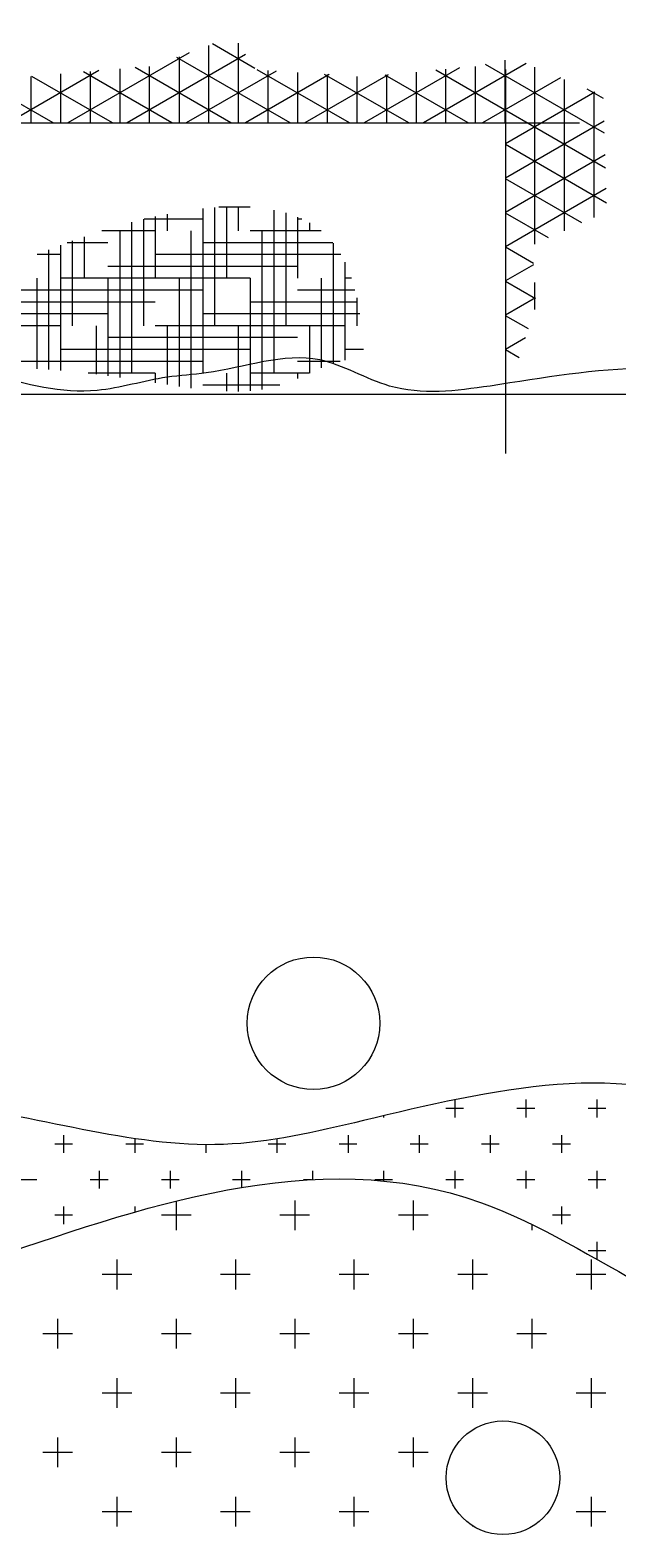
# Model space of a CAD drawing. Units: inches. Extents: x 3731 to 4318, y 1310 to 2388.
# Tile 45 of 57: x 4167 to 4192, y 1977 to 2043. Entities that reach past the tile are written whole.
import ezdxf

# ---------------------------------------------------------------- set-up
doc = ezdxf.new("R2010")
doc.units = ezdxf.units.IN
doc.layers.add('A-ANNO-DIMS', color=2, linetype='Continuous', lineweight=18)
doc.layers.add('A-FURN', color=8, linetype='Continuous', lineweight=13)
doc.styles.get("Standard").update_dxf_attribs({"font": 'arial.ttf'})
doc.dimstyles.get("Standard").update_dxf_attribs({"dimtxt": 0.18, "dimasz": 0.18, "dimexe": 0.18, "dimexo": 0.0625, "dimgap": 0.09, "dimtad": 0, "dimtih": 1, "dimtoh": 1, "dimdec": 4, "dimzin": 0, "dimdsep": 46, "dimtxsty": 'Standard', "dimcen": 0.09, "dimadec": 0, "dimazin": 0, "dimtfac": 1, "dimtdec": 4, "dimtofl": 0, "dimtmove": 0, "dimatfit": 3, "dimfxl": 1, "dimtolj": 1, "dimtzin": 0, "dimarcsym": 0})

# ---------------------------------------------------------------- blocks, each defined once
blk = doc.blocks.new('A$C200C7901')
at = {"linetype": 'ByBlock'}
for p, q in [((0.9504, 1.532), (0.9504, 1.5633)), ((0.9504, 1.532), (0.9504, 1.5633)), ((1.2004, 1.532), (1.2004, 1.5633)), ((1.2004, 1.532), (1.2004, 1.5633)), ((1.3254, 1.532), (1.3254, 1.5633)), ((1.3254, 1.532), (1.3254, 1.5633)), ((1.4504, 1.532), (1.4504, 1.5633)), ((1.4504, 1.532), (1.4504, 1.5633)), ((0.9347, 1.5477), (0.966, 1.5477)), ((0.9347, 1.5477), (0.966, 1.5477)), ((1.1847, 1.5477), (1.216, 1.5477)), ((1.1847, 1.5477), (1.216, 1.5477)), ((1.3097, 1.5477), (1.341, 1.5477)), ((1.3097, 1.5477), (1.341, 1.5477)), ((1.4347, 1.5477), (1.466, 1.5477)), ((1.4347, 1.5477), (1.466, 1.5477)), ((1.1379, 1.4695), (1.1379, 1.5008)), ((1.1379, 1.4695), (1.1379, 1.5008)), ((1.2629, 1.4695), (1.2629, 1.5008)), ((1.2629, 1.4695), (1.2629, 1.5008)), ((1.3879, 1.4695), (1.3879, 1.5008)), ((1.3879, 1.4695), (1.3879, 1.5008)), ((1.5129, 1.4695), (1.5129, 1.5008)), ((1.5129, 1.4695), (1.5129, 1.5008)), ((1.1222, 1.4852), (1.1535, 1.4852)), ((1.1222, 1.4852), (1.1535, 1.4852)), ((1.2472, 1.4852), (1.2785, 1.4852)), ((1.2472, 1.4852), (1.2785, 1.4852)), ((1.3722, 1.4852), (1.4035, 1.4852)), ((1.3722, 1.4852), (1.4035, 1.4852)), ((1.4972, 1.4852), (1.5285, 1.4852)), ((1.4972, 1.4852), (1.5285, 1.4852)), ((0.9504, 1.407), (0.9504, 1.4383)), ((0.9504, 1.407), (0.9504, 1.4383)), ((1.0754, 1.407), (1.0754, 1.4383)), ((1.0754, 1.407), (1.0754, 1.4383)), ((1.2004, 1.407), (1.2004, 1.4383)), ((1.2004, 1.407), (1.2004, 1.4383)), ((1.3254, 1.407), (1.3254, 1.4383)), ((1.3254, 1.407), (1.3254, 1.4383)), ((1.4504, 1.407), (1.4504, 1.4383)), ((1.4504, 1.407), (1.4504, 1.4383)), ((0.9347, 1.4227), (0.966, 1.4227)), ((0.9347, 1.4227), (0.966, 1.4227)), ((1.0597, 1.4227), (1.091, 1.4227)), ((1.0597, 1.4227), (1.091, 1.4227)), ((1.1847, 1.4227), (1.216, 1.4227)), ((1.1847, 1.4227), (1.216, 1.4227)), ((1.3097, 1.4227), (1.341, 1.4227)), ((1.3097, 1.4227), (1.341, 1.4227)), ((1.4347, 1.4227), (1.466, 1.4227)), ((1.4347, 1.4227), (1.466, 1.4227)), ((1.0129, 1.3445), (1.0129, 1.3758)), ((1.0129, 1.3445), (1.0129, 1.3758)), ((1.1379, 1.3445), (1.1379, 1.3758)), ((1.1379, 1.3445), (1.1379, 1.3758)), ((1.2629, 1.3445), (1.2629, 1.3758)), ((1.2629, 1.3445), (1.2629, 1.3758)), ((1.3879, 1.3445), (1.3879, 1.3758)), ((1.3879, 1.3445), (1.3879, 1.3758)), ((1.5129, 1.3445), (1.5129, 1.3758)), ((1.5129, 1.3445), (1.5129, 1.3758)), ((0.9972, 1.3602), (1.0285, 1.3602)), ((0.9972, 1.3602), (1.0285, 1.3602)), ((1.1222, 1.3602), (1.1535, 1.3602)), ((1.1222, 1.3602), (1.1535, 1.3602)), ((1.2472, 1.3602), (1.2785, 1.3602)), ((1.2472, 1.3602), (1.2785, 1.3602)), ((1.3722, 1.3602), (1.4035, 1.3602)), ((1.3722, 1.3602), (1.4035, 1.3602)), ((1.4972, 1.3602), (1.5285, 1.3602)), ((1.4972, 1.3602), (1.5285, 1.3602)), ((0.9504, 1.282), (0.9504, 1.3133)), ((0.9504, 1.282), (0.9504, 1.3133)), ((1.0754, 1.282), (1.0754, 1.3133)), ((1.0754, 1.282), (1.0754, 1.3133)), ((1.2004, 1.282), (1.2004, 1.3133)), ((1.2004, 1.282), (1.2004, 1.3133)), ((1.3254, 1.282), (1.3254, 1.3133)), ((1.3254, 1.282), (1.3254, 1.3133)), ((1.4504, 1.282), (1.4504, 1.3133)), ((1.4504, 1.282), (1.4504, 1.3133)), ((0.9347, 1.2977), (0.966, 1.2977)), ((0.9347, 1.2977), (0.966, 1.2977)), ((1.0597, 1.2977), (1.091, 1.2977)), ((1.0597, 1.2977), (1.091, 1.2977)), ((1.1847, 1.2977), (1.216, 1.2977)), ((1.1847, 1.2977), (1.216, 1.2977)), ((1.3097, 1.2977), (1.341, 1.2977)), ((1.3097, 1.2977), (1.341, 1.2977)), ((1.4347, 1.2977), (1.466, 1.2977)), ((1.4347, 1.2977), (1.466, 1.2977)), ((0.9347, 1.2727), (0.9535, 1.2727)), ((0.9347, 1.2727), (0.9535, 1.2727)), ((0.9441, 1.2633), (0.9441, 1.2816)), ((0.9441, 1.2633), (0.9441, 1.2816)), ((0.9816, 1.2258), (0.9816, 1.2445)), ((0.9816, 1.2258), (0.9816, 1.2445)), ((1.0129, 1.2448), (1.0129, 1.2508)), ((1.0129, 1.2448), (1.0129, 1.2508)), ((1.1379, 1.2195), (1.1379, 1.2508)), ((1.1379, 1.2195), (1.1379, 1.2508)), ((1.2629, 1.2195), (1.2629, 1.2508)), ((1.2629, 1.2195), (1.2629, 1.2508)), ((1.3879, 1.2202), (1.3879, 1.2508)), ((1.3879, 1.2202), (1.3879, 1.2508)), ((1.5066, 1.2258), (1.5066, 1.2445)), ((1.5066, 1.2258), (1.5066, 1.2445)), ((0.9722, 1.2352), (0.991, 1.2352)), ((0.9722, 1.2352), (0.991, 1.2352)), ((1.1222, 1.2352), (1.1535, 1.2352)), ((1.1222, 1.2352), (1.1535, 1.2352)), ((1.2472, 1.2352), (1.2785, 1.2352)), ((1.2472, 1.2352), (1.2785, 1.2352)), ((1.3722, 1.2352), (1.4035, 1.2352)), ((1.3722, 1.2352), (1.4035, 1.2352)), ((1.4316, 1.2258), (1.4316, 1.2318)), ((1.4316, 1.2258), (1.4316, 1.2318)), ((1.4972, 1.2352), (1.516, 1.2352)), ((1.4972, 1.2352), (1.516, 1.2352)), ((0.9347, 1.1977), (0.9535, 1.1977)), ((0.9347, 1.1977), (0.9535, 1.1977)), ((0.9441, 1.1883), (0.9441, 1.207)), ((0.9441, 1.1883), (0.9441, 1.207)), ((1.0097, 1.1977), (1.0285, 1.1977)), ((1.0097, 1.1977), (1.0285, 1.1977)), ((1.0191, 1.1883), (1.0191, 1.207)), ((1.0191, 1.1883), (1.0191, 1.207)), ((1.0847, 1.1977), (1.1035, 1.1977)), ((1.0847, 1.1977), (1.1035, 1.1977)), ((1.0941, 1.1883), (1.0941, 1.207)), ((1.0941, 1.1883), (1.0941, 1.207)), ((1.1597, 1.1977), (1.1785, 1.1977)), ((1.1597, 1.1977), (1.1785, 1.1977)), ((1.1691, 1.1883), (1.1691, 1.1991)), ((1.1691, 1.1883), (1.1691, 1.1991)), ((1.2441, 1.1883), (1.2441, 1.1976)), ((1.2441, 1.1883), (1.2441, 1.1976)), ((1.2452, 1.1977), (1.2535, 1.1977)), ((1.2452, 1.1977), (1.2535, 1.1977)), ((1.3097, 1.1977), (1.3285, 1.1977)), ((1.3097, 1.1977), (1.3285, 1.1977)), ((1.3191, 1.1883), (1.3191, 1.2059)), ((1.3191, 1.1883), (1.3191, 1.2059)), ((1.3847, 1.1977), (1.4035, 1.1977)), ((1.3847, 1.1977), (1.4035, 1.1977)), ((1.3941, 1.1883), (1.3941, 1.207)), ((1.3941, 1.1883), (1.3941, 1.207)), ((1.4597, 1.1977), (1.4785, 1.1977)), ((1.4597, 1.1977), (1.4785, 1.1977)), ((1.4691, 1.1883), (1.4691, 1.207)), ((1.4691, 1.1883), (1.4691, 1.207)), ((1.5347, 1.1977), (1.5535, 1.1977)), ((1.5347, 1.1977), (1.5535, 1.1977)), ((0.9722, 1.1602), (0.991, 1.1602)), ((0.9722, 1.1602), (0.991, 1.1602)), ((0.9816, 1.1508), (0.9816, 1.1695)), ((0.9816, 1.1508), (0.9816, 1.1695)), ((1.0472, 1.1602), (1.066, 1.1602)), ((1.0472, 1.1602), (1.066, 1.1602)), ((1.0566, 1.1508), (1.0566, 1.1695)), ((1.0566, 1.1508), (1.0566, 1.1695)), ((1.1222, 1.1602), (1.141, 1.1602)), ((1.1222, 1.1602), (1.141, 1.1602)), ((1.1316, 1.1508), (1.1316, 1.1695)), ((1.1316, 1.1508), (1.1316, 1.1695)), ((1.1972, 1.1602), (1.216, 1.1602)), ((1.1972, 1.1602), (1.216, 1.1602)), ((1.2066, 1.1508), (1.2066, 1.1695)), ((1.2066, 1.1508), (1.2066, 1.1695)), ((1.2722, 1.1602), (1.291, 1.1602)), ((1.2722, 1.1602), (1.291, 1.1602)), ((1.2816, 1.1547), (1.2816, 1.1695)), ((1.2816, 1.1547), (1.2816, 1.1695)), ((1.3566, 1.1608), (1.3566, 1.1695)), ((1.3566, 1.1608), (1.3566, 1.1695)), ((1.4222, 1.1602), (1.441, 1.1602)), ((1.4222, 1.1602), (1.441, 1.1602)), ((1.4316, 1.1544), (1.4316, 1.1695)), ((1.4316, 1.1544), (1.4316, 1.1695)), ((1.4972, 1.1602), (1.516, 1.1602)), ((1.4972, 1.1602), (1.516, 1.1602)), ((1.5066, 1.1508), (1.5066, 1.1695)), ((1.5066, 1.1508), (1.5066, 1.1695)), ((0.9441, 1.1133), (0.9441, 1.132)), ((0.9441, 1.1133), (0.9441, 1.132)), ((1.0191, 1.1133), (1.0191, 1.132)), ((1.0191, 1.1133), (1.0191, 1.132)), ((1.0941, 1.1136), (1.0941, 1.132)), ((1.0941, 1.1136), (1.0941, 1.132)), ((1.1691, 1.1303), (1.1691, 1.132)), ((1.1691, 1.1303), (1.1691, 1.132)), ((0.9347, 1.1227), (0.9535, 1.1227)), ((0.9347, 1.1227), (0.9535, 1.1227)), ((1.0097, 1.1227), (1.0285, 1.1227)), ((1.0097, 1.1227), (1.0285, 1.1227)), ((1.0847, 1.1227), (1.1035, 1.1227)), ((1.0847, 1.1227), (1.1035, 1.1227)), ((1.3099, 0.2477), (1.3099, 0.3663)), ((1.3099, 0.2477), (1.3099, 0.3663)), ((1.3224, 0.2977), (1.3224, 0.3669)), ((1.3224, 0.2977), (1.3224, 0.3669)), ((1.3349, 0.3477), (1.3349, 0.3668)), ((1.3349, 0.3477), (1.3349, 0.3668)), ((1.2599, 0.3477), (1.2599, 0.3531)), ((1.2599, 0.3477), (1.2599, 0.3531)), ((1.2785, 0.3602), (1.3599, 0.3602)), ((1.2785, 0.3602), (1.3599, 0.3602)), ((1.2974, 0.1977), (1.2974, 0.3647)), ((1.2974, 0.1977), (1.2974, 0.3647)), ((1.3724, 0.1977), (1.3724, 0.3634)), ((1.3724, 0.1977), (1.3724, 0.3634)), ((1.3849, 0.2477), (1.3849, 0.3616)), ((1.3849, 0.2477), (1.3849, 0.3616)), ((1.3974, 0.2977), (1.3974, 0.3597)), ((1.3974, 0.2977), (1.3974, 0.3597)), ((1.4099, 0.3477), (1.4099, 0.3578)), ((1.4099, 0.3477), (1.4099, 0.3578)), ((1.4474, 0.1977), (1.4474, 0.3521)), ((1.4474, 0.1977), (1.4474, 0.3521)), ((1.4599, 0.2477), (1.4599, 0.3504)), ((1.4599, 0.2477), (1.4599, 0.3504)), ((1.2099, 0.2308), (1.2099, 0.334)), ((1.2099, 0.2308), (1.2099, 0.334)), ((1.2148, 0.3352), (1.2599, 0.3352)), ((1.2148, 0.3352), (1.2599, 0.3352)), ((1.2224, 0.2106), (1.2224, 0.3375)), ((1.2224, 0.2106), (1.2224, 0.3375)), ((1.2349, 0.2477), (1.2349, 0.3422)), ((1.2349, 0.2477), (1.2349, 0.3422)), ((1.2474, 0.2977), (1.2474, 0.3476)), ((1.2474, 0.2977), (1.2474, 0.3476)), ((1.2475, 0.3477), (1.3099, 0.3477)), ((1.2475, 0.3477), (1.3099, 0.3477)), ((1.2849, 0.1758), (1.2849, 0.3477)), ((1.2849, 0.1758), (1.2849, 0.3477)), ((1.3599, 0.1741), (1.3599, 0.3477)), ((1.3599, 0.1741), (1.3599, 0.3477)), ((1.3599, 0.3352), (1.5599, 0.3352)), ((1.3599, 0.3352), (1.5599, 0.3352)), ((1.4099, 0.3477), (1.4806, 0.3477)), ((1.4099, 0.3477), (1.4806, 0.3477)), ((1.4349, 0.1886), (1.4349, 0.3477)), ((1.4349, 0.1886), (1.4349, 0.3477)), ((1.4724, 0.2977), (1.4724, 0.3487)), ((1.4724, 0.2977), (1.4724, 0.3487)), ((1.5099, 0.2129), (1.5099, 0.3447)), ((1.5099, 0.2129), (1.5099, 0.3447)), ((1.5224, 0.2177), (1.5224, 0.3438)), ((1.5224, 0.2177), (1.5224, 0.3438)), ((1.5349, 0.2477), (1.5349, 0.3431)), ((1.5349, 0.2477), (1.5349, 0.3431)), ((1.0194, 0.3103), (1.0407, 0.3227)), ((1.0194, 0.3103), (1.0407, 0.3227)), ((1.0261, 0.3316), (1.0407, 0.3232)), ((1.0261, 0.3316), (1.0407, 0.3232)), ((1.1904, 0.3227), (1.2099, 0.3227)), ((1.1904, 0.3227), (1.2099, 0.3227)), ((1.3099, 0.3227), (1.5099, 0.3227)), ((1.3099, 0.3227), (1.5099, 0.3227)), ((1.2599, 0.3102), (1.4599, 0.3102)), ((1.2599, 0.3102), (1.4599, 0.3102)), ((1.0089, 0.2682), (1.0407, 0.2866)), ((1.0089, 0.2682), (1.0407, 0.2866)), ((1.0164, 0.3011), (1.0407, 0.2871)), ((1.0164, 0.3011), (1.0407, 0.2871)), ((1.1974, 0.2683), (1.1974, 0.2977)), ((1.1974, 0.2683), (1.1974, 0.2977)), ((1.2099, 0.2977), (1.4099, 0.2977)), ((1.2099, 0.2977), (1.4099, 0.2977)), ((1.2724, 0.1788), (1.2724, 0.2977)), ((1.2724, 0.1788), (1.2724, 0.2977)), ((1.3474, 0.173), (1.3474, 0.2977)), ((1.3474, 0.173), (1.3474, 0.2977)), ((1.4224, 0.1854), (1.4224, 0.2977)), ((1.4224, 0.1854), (1.4224, 0.2977)), ((1.4974, 0.2083), (1.4974, 0.2977)), ((1.4974, 0.2083), (1.4974, 0.2977)), ((1.5099, 0.2977), (1.7099, 0.2977)), ((1.5099, 0.2977), (1.7099, 0.2977)), ((1.0099, 0.2521), (1.0099, 0.2804)), ((1.0099, 0.2521), (1.0099, 0.2804)), ((1.1943, 0.2852), (1.3599, 0.2852)), ((1.1943, 0.2852), (1.3599, 0.2852)), ((1.1965, 0.2727), (1.3099, 0.2727)), ((1.1965, 0.2727), (1.3099, 0.2727)), ((1.4099, 0.2727), (1.6099, 0.2727)), ((1.4099, 0.2727), (1.6099, 0.2727)), ((1.4599, 0.2852), (1.6599, 0.2852)), ((1.4599, 0.2852), (1.6599, 0.2852)), ((1.0088, 0.2694), (1.0407, 0.251)), ((1.0088, 0.2694), (1.0407, 0.251)), ((1.1994, 0.2602), (1.2599, 0.2602)), ((1.1994, 0.2602), (1.2599, 0.2602)), ((1.3599, 0.2602), (1.5599, 0.2602)), ((1.3599, 0.2602), (1.5599, 0.2602)), ((1.0111, 0.2334), (1.0407, 0.2505)), ((1.0111, 0.2334), (1.0407, 0.2505)), ((1.2031, 0.2477), (1.2099, 0.2477)), ((1.2031, 0.2477), (1.2099, 0.2477)), ((1.2599, 0.1831), (1.2599, 0.2477)), ((1.2599, 0.1831), (1.2599, 0.2477)), ((1.3099, 0.2477), (1.5099, 0.2477)), ((1.3099, 0.2477), (1.5099, 0.2477)), ((1.3349, 0.1723), (1.3349, 0.2477)), ((1.3349, 0.1723), (1.3349, 0.2477)), ((1.4099, 0.1825), (1.4099, 0.2477)), ((1.4099, 0.1825), (1.4099, 0.2477)), ((1.4849, 0.2039), (1.4849, 0.2477)), ((1.4849, 0.2039), (1.4849, 0.2477)), ((1.0112, 0.232), (1.0407, 0.215)), ((1.0112, 0.232), (1.0407, 0.215)), ((1.2142, 0.2227), (1.4099, 0.2227)), ((1.2142, 0.2227), (1.4099, 0.2227)), ((1.2599, 0.2352), (1.4599, 0.2352)), ((1.2599, 0.2352), (1.4599, 0.2352)), ((1.5099, 0.2227), (1.5346, 0.2227)), ((1.5099, 0.2227), (1.5346, 0.2227)), ((0.9344, 0.153), (1.0407, 0.2144)), ((0.9344, 0.153), (1.0407, 0.2144)), ((1.0099, 0.0251), (1.0099, 0.2117)), ((1.0099, 0.0251), (1.0099, 0.2117)), ((1.2227, 0.2102), (1.3599, 0.2102)), ((1.2227, 0.2102), (1.3599, 0.2102)), ((1.4599, 0.2102), (1.5027, 0.2102)), ((1.4599, 0.2102), (1.5027, 0.2102)), ((0.9787, 0.0381), (0.9787, 0.1976)), ((0.9787, 0.0381), (0.9787, 0.1976)), ((0.9953, 0.2051), (1.0407, 0.1789)), ((0.9953, 0.2051), (1.0407, 0.1789)), ((1.2351, 0.1977), (1.3099, 0.1977)), ((1.2351, 0.1977), (1.3099, 0.1977)), ((1.2474, 0.1892), (1.2474, 0.1977)), ((1.2474, 0.1892), (1.2474, 0.1977)), ((1.3224, 0.1722), (1.3224, 0.1977)), ((1.3224, 0.1722), (1.3224, 0.1977)), ((1.3974, 0.1799), (1.3974, 0.1977)), ((1.3974, 0.1799), (1.3974, 0.1977)), ((1.4099, 0.1977), (1.4662, 0.1977)), ((1.4099, 0.1977), (1.4662, 0.1977)), ((0.9355, 0.1176), (1.0407, 0.1783)), ((0.9355, 0.1176), (1.0407, 0.1783)), ((0.9474, 0.0512), (0.9474, 0.1835)), ((0.9474, 0.0512), (0.9474, 0.1835)), ((0.9602, 0.1893), (1.0407, 0.1428)), ((0.9602, 0.1893), (1.0407, 0.1428)), ((1.2552, 0.1852), (1.2599, 0.1852)), ((1.2552, 0.1852), (1.2599, 0.1852)), ((1.3599, 0.1852), (1.4215, 0.1852)), ((1.3599, 0.1852), (1.4215, 0.1852)), ((0.9339, 0.1684), (1.0407, 0.1067)), ((0.9339, 0.1684), (1.0407, 0.1067)), ((1.3099, 0.1727), (1.3428, 0.1727)), ((1.3099, 0.1727), (1.3428, 0.1727)), ((0.935, 0.1316), (1.114, 0.0283)), ((0.935, 0.1316), (1.114, 0.0283)), ((0.9366, 0.0822), (1.0407, 0.1422)), ((0.9366, 0.0822), (1.0407, 0.1422)), ((0.9463, 0.0516), (1.0407, 0.1061)), ((0.9463, 0.0516), (1.0407, 0.1061)), ((0.9362, 0.0948), (1.0616, 0.0225)), ((0.9362, 0.0948), (1.0616, 0.0225)), ((0.9826, 0.0365), (1.0647, 0.0839)), ((0.9826, 0.0365), (1.0647, 0.0839)), ((1.0189, 0.0214), (1.1272, 0.0839)), ((1.0189, 0.0214), (1.1272, 0.0839)), ((1.0412, 0.0179), (1.0412, 0.0839)), ((1.0412, 0.0179), (1.0412, 0.0839)), ((1.0724, 0.0243), (1.0724, 0.0839)), ((1.0724, 0.0243), (1.0724, 0.0839)), ((1.0801, 0.0839), (1.1675, 0.0335)), ((1.0801, 0.0839), (1.1675, 0.0335)), ((1.0891, 0.0259), (1.1897, 0.0839)), ((1.0891, 0.0259), (1.1897, 0.0839)), ((1.1037, 0.0273), (1.1037, 0.0839)), ((1.1037, 0.0273), (1.1037, 0.0839)), ((1.1349, 0.0303), (1.1349, 0.0839)), ((1.1349, 0.0303), (1.1349, 0.0839)), ((1.1426, 0.0839), (1.2313, 0.0327)), ((1.1426, 0.0839), (1.2313, 0.0327)), ((1.1642, 0.0331), (1.2522, 0.0839)), ((1.1642, 0.0331), (1.2522, 0.0839)), ((1.1662, 0.0333), (1.1662, 0.0839)), ((1.1662, 0.0333), (1.1662, 0.0839)), ((1.1974, 0.0351), (1.1974, 0.0839)), ((1.1974, 0.0351), (1.1974, 0.0839)), ((1.2051, 0.0839), (1.3023, 0.0278)), ((1.2051, 0.0839), (1.3023, 0.0278)), ((1.2266, 0.033), (1.3147, 0.0839)), ((1.2266, 0.033), (1.3147, 0.0839)), ((1.2287, 0.0329), (1.2287, 0.0839)), ((1.2287, 0.0329), (1.2287, 0.0839)), ((1.2599, 0.0308), (1.2599, 0.0839)), ((1.2599, 0.0308), (1.2599, 0.0839)), ((1.2676, 0.0839), (1.3871, 0.015)), ((1.2676, 0.0839), (1.3871, 0.015)), ((1.2824, 0.0292), (1.3772, 0.0839)), ((1.2824, 0.0292), (1.3772, 0.0839)), ((1.2912, 0.0286), (1.2912, 0.0839)), ((1.2912, 0.0286), (1.2912, 0.0839)), ((1.3146, 0.0117), (1.4397, 0.0839)), ((1.3146, 0.0117), (1.4397, 0.0839)), ((1.3224, 0), (1.3224, 0.0839)), ((1.3224, 0), (1.3224, 0.0839)), ((1.3301, 0.0839), (1.4312, 0.0256)), ((1.3301, 0.0839), (1.4312, 0.0256)), ((1.3537, 0.0022), (1.3537, 0.0839)), ((1.3537, 0.0022), (1.3537, 0.0839)), ((1.3743, 0.0101), (1.5022, 0.0839)), ((1.3743, 0.0101), (1.5022, 0.0839)), ((1.3849, 0.0141), (1.3849, 0.0839)), ((1.3849, 0.0141), (1.3849, 0.0839)), ((1.3926, 0.0839), (1.4856, 0.0302)), ((1.3926, 0.0839), (1.4856, 0.0302)), ((1.4162, 0.0243), (1.4162, 0.0839)), ((1.4162, 0.0243), (1.4162, 0.0839)), ((1.4474, 0.027), (1.4474, 0.0839)), ((1.4474, 0.027), (1.4474, 0.0839)), ((1.4551, 0.0839), (1.54, 0.0349)), ((1.4551, 0.0839), (1.54, 0.0349)), ((1.4693, 0.0288), (1.5647, 0.0839)), ((1.4693, 0.0288), (1.5647, 0.0839)), ((1.4787, 0.0296), (1.4787, 0.0839)), ((1.4787, 0.0296), (1.4787, 0.0839)), ((1.5099, 0.0323), (1.5099, 0.0839)), ((1.5099, 0.0323), (1.5099, 0.0839)), ((1.5176, 0.0839), (1.6251, 0.0219)), ((1.5176, 0.0839), (1.6251, 0.0219)), ((1.5412, 0.035), (1.5412, 0.0839)), ((1.5412, 0.035), (1.5412, 0.0839)), ((0.9374, 0.0581), (0.9545, 0.0482)), ((0.9374, 0.0581), (0.9545, 0.0482)), ((1.3048, 0.0264), (1.3494, 0.0006)), ((1.3048, 0.0264), (1.3494, 0.0006))]:
    blk.add_line(p, q, dxfattribs=at)
for p, q in [((1.0754, 1.5625), (1.0754, 1.5633)), ((1.0754, 1.5625), (1.0754, 1.5633)), ((1.0407, 0.0275), (1.0407, 0.4323)), ((0.4061, 0.3703), (2.0386, 0.3703)), ((2.4073, 0.0839), (0.9625, 0.0839))]:
    blk.add_line(p, q)
for centre, radius in [((1.0433, 1.5119), 0.0599), ((1.2431, 1.0329), 0.0699)]:
    blk.add_circle(centre, radius)
for points, knots in [([(0.4485, 1.7835), (0.4321, 1.7496), (0.4062, 1.6964), (0.49, 1.6713), (0.4719, 1.5969), (0.4123, 1.592), (0.4233, 1.5337), (0.4954, 1.5086), (0.4012, 1.4738), (0.3253, 1.4306), (0.4113, 1.3764), (0.3688, 1.3065), (0.5579, 1.2663), (0.741, 1.4533), (1.1127, 1.1109), (1.4811, 1.2478), (1.7885, 1.3492), (2.0357, 1.1637), (2.0748, 1.2974), (2.0876, 1.349), (2.0192, 1.3805), (2.0564, 1.4298), (2.0588, 1.4846), (1.9759, 1.5349), (2.1004, 1.5845), (2.0397, 1.6519), (1.971, 1.7053), (2.1104, 1.8981), (1.5946, 1.7967), (1.2448, 1.7472), (0.8129, 1.7935), (0.4953, 1.8548), (0.4582, 1.7983), (0.4485, 1.7835)], [0, 0, 0, 0, 88.420092, 139.08588, 204.302936, 239.695496, 287.801042, 327.365471, 412.960499, 463.626286, 552.059846, 584.668336, 662.614915, 940.993281, 1309.926334, 1844.022653, 1996.276242, 2316.43048, 2341.441004, 2404.707416, 2449.463774, 2514.680778, 2538.40571, 2613.031547, 2697.13096, 2760.903931, 2822.692699, 2945.47, 3215.060018, 3725.584917, 4361.974444, 4504.671998, 4555.32777, 4555.32777, 4555.32777, 4555.32777]), ([(0.4856, 1.3429), (0.5504, 1.3182), (0.6715, 1.2721), (0.8374, 1.0498), (1.1164, 1.1183), (1.3878, 1.1816), (1.5888, 1.1102), (1.8403, 1.1127), (1.9415, 1.2178), (2.0032, 1.2819)], [0, 0, 0, 0, 205.411753, 383.654933, 772.067458, 921.644661, 1226.793228, 1388.983508, 1642.292305, 1642.292305, 1642.292305, 1642.292305])]:
    blk.add_open_spline(points, degree=3, knots=knots)
blk.add_open_spline([(0.473, 1.2954), (0.4739, 1.2781), (0.4755, 1.2477), (0.5032, 1.2084), (0.4801, 1.1701), (0.4928, 1.1255), (0.4674, 1.0912), (0.4579, 1.0351), (0.501, 0.9724), (0.4311, 0.8832), (0.4902, 0.8637), (0.4843, 0.8288), (0.4774, 0.7906), (0.4625, 0.7457), (0.459, 0.6999), (0.4816, 0.6664), (0.4748, 0.625), (0.4791, 0.5889), (0.4533, 0.5528), (0.4738, 0.5004), (0.4658, 0.4502), (0.4696, 0.3946), (0.4189, 0.3935), (0.4493, 0.3684), (0.4694, 0.3857), (0.4922, 0.3576), (0.5297, 0.3262), (0.5917, 0.3353), (0.6454, 0.3754), (0.7083, 0.3741), (0.7643, 0.3328), (0.826, 0.346), (0.925, 0.3388), (1.0353, 0.3593), (1.1561, 0.3744), (1.2477, 0.3154), (1.3302, 0.3474), (1.4086, 0.3512), (1.5217, 0.3878), (1.6362, 0.3176), (1.7682, 0.3285), (1.8402, 0.3019), (1.9071, 0.3529), (1.9647, 0.3412), (2.0795, 0.2948), (2.0472, 0.3498), (2.0343, 0.3772), (2.0435, 0.43), (2.0109, 0.5782), (2.0746, 0.4643), (2.0805, 0.584), (2.0084, 0.5979), (2.0343, 0.6846), (2.0344, 0.746), (2.0293, 0.8096), (2.0489, 0.8545), (2.0652, 0.9218), (1.9842, 0.9297), (2.0007, 1.0162), (2.0367, 1.0585), (2.0367, 1.1102), (2.0457, 1.1647), (2.0226, 1.2084), (2.0234, 1.2306), (2.0236, 1.2352)], degree=3, knots=[0, 0, 0, 0, 51.660678, 90.967412, 128.902454, 170.303599, 219.852997, 247.834962, 336.321557, 429.35469, 458.821847, 477.222321, 524.135809, 581.038434, 617.839381, 657.146115, 693.947125, 740.178081, 760.753248, 820.731705, 885.133458, 928.777044, 953.563729, 976.574207, 995.553042, 1018.563482, 1064.584401, 1147.951297, 1174.787598, 1266.851571, 1308.018447, 1377.066427, 1441.511314, 1608.245014, 1714.11869, 1792.771707, 1913.247991, 1954.931389, 2029.864445, 2259.189419, 2305.221512, 2429.507982, 2456.344283, 2543.92595, 2627.925037, 2662.96218, 2687.736879, 2719.937755, 2839.540991, 2875.47895, 2953.681041, 2993.270313, 3066.872333, 3154.395764, 3200.397042, 3248.426375, 3312.828127, 3347.881398, 3444.484026, 3481.577522, 3518.665244, 3592.267265, 3644.719162, 3658.519501, 3658.519501, 3658.519501, 3658.519501], dxfattribs=at)
blk = doc.blocks.new('*D38')
at = {"layer": 'A-ANNO-DIMS', "color": 0, "lineweight": -2, "transparency": 16777216}
for p, q in [((4103.271, 2262.382), (4318.341, 2262.382)), ((4318.161, 2262.202), (4318.161, 2103.064)), ((4318.161, 1943.562), (4318.161, 2102.7)), ((4234.271, 1943.382), (4318.341, 1943.382))]:
    blk.add_line(p, q, dxfattribs=at)
at = {"layer": 'A-ANNO-DIMS', "color": 0, "transparency": 16777216}
for points in [[(4318.131, 2262.202), (4318.191, 2262.202), (4318.161, 2262.382)], [(4318.131, 1943.562), (4318.191, 1943.562), (4318.161, 1943.382)]]:
    blk.add_solid(points, dxfattribs=at)
at = {"layer": 'Defpoints', "color": 0, "transparency": 16777216}
for p in [(4103.209, 2262.382), (4318.161, 2262.382), (4234.209, 1943.382)]:
    blk.add_point(p, dxfattribs=at)
at = {"layer": 'A-ANNO-DIMS', "color": 0, "transparency": 16777216, "insert": (4318.161, 2102.882), "char_height": 0.18, "attachment_point": 5}
blk.add_mtext('\\A1;319', dxfattribs=at)

msp = doc.modelspace()

# ---------------------------------------------------------------- block references
at = {"layer": 'A-FURN', "xscale": 41.1071563136412, "yscale": 41.1071563136412, "zscale": 41.1071563136412, "rotation": 180}
msp.add_blockref('A$C200C7901', (4230.145, 2042.037), dxfattribs=at)

# ---------------------------------------------------------------- dimensions: what is measured, and where the dimension line sits
at = {"layer": 'A-ANNO-DIMS'}
dim = msp.add_linear_dim(base=(4318.161, 2262.382), p1=(4234.209, 1943.382), p2=(4103.209, 2262.382), angle=90, dimstyle='Standard', override={"dimdec": 0, "dimlfac": 1, "dimrnd": 0, "dimzin": 0, "dimdsep": 46, "dimlunit": 2}, dxfattribs=at)
dim.commit()
dim.dimension.update_dxf_attribs({"geometry": '*D38', "text_midpoint": (4318.161, 2102.882)})

doc.saveas('drawing.dxf')
